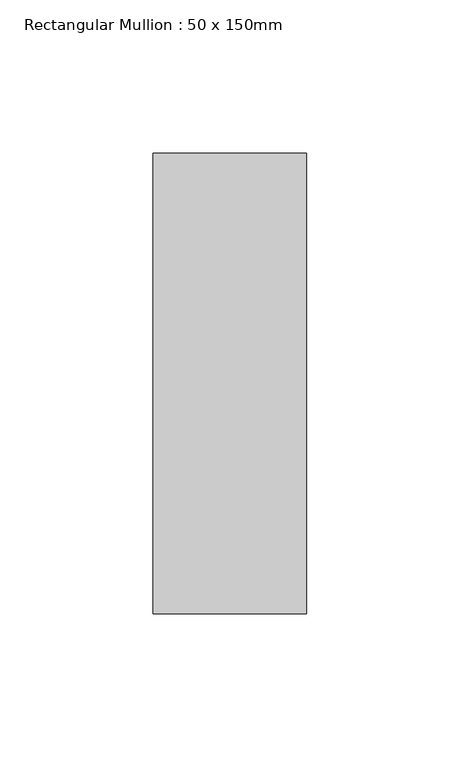
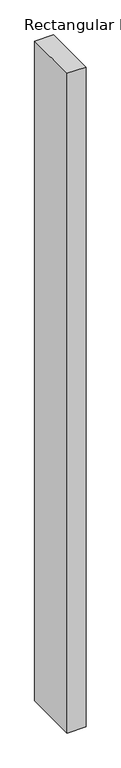
"""IFC4 building model written with IfcOpenShell, lengths in millimetres: member geometry, Rectangular Mullion : 50 x 150mm."""

from ifc_helpers import new_model, si_unit, frame, origin, place, context, project, spatial, polyline, outline, extrude, source, transform, mapped, element, save


def rectangular_mullion_50_x_150mm_17218063(model_context):
    return source(origin(), model_context, "Body", "SweptSolid", [
        extrude(outline(polyline([(0.0, 75.0), (0.0, -75.0), (-50.0, -75.0), (-50.0, 75.0), (0.0, 75.0)])), frame((0.0, 0.0, -1855.0), z_axis=(0.0, 0.0, 1.0), x_axis=(1.0, 0.0, 0.0)), (0.0, 0.0, 1.0), 1855.0),
    ])


if __name__ == "__main__":
    model = new_model("IFC4")
    model_context = context("Model", 3, world=origin())
    ifc_project = project(units=[si_unit("LENGTHUNIT", "METRE", prefix="MILLI")], contexts=[model_context])
    site = spatial("IfcSite", under=ifc_project)
    building = spatial("IfcBuilding", under=site)
    placement = place(None, origin())
    rectangular_mullion_50_x_150mm_shape = rectangular_mullion_50_x_150mm_17218063(model_context)
    element("IfcMember", 1, ObjectType="Rectangular Mullion : 50 x 150mm", at=placement, inside=building, context=model_context, shape_type="MappedRepresentation", body=[
        mapped(rectangular_mullion_50_x_150mm_shape, transform((0.0, 0.0, 0.0), x_axis=(1.0, 0.0, 0.0), y_axis=(0.0, 1.0, 0.0), z_axis=(0.0, 0.0, 1.0))),
    ])
    save(model, "model.ifc")

# Revit data of these elements
# Type "Rectangular Mullion : 50 x 150mm"
#   built-in parameter 1007304 = 0.492126 (stored number, unit not read)
#   built-in parameter 1007301 = 0.082021 (stored number, unit not read)
#   built-in parameter 1007300 = 0.082021 (stored number, unit not read)
# Element 1 (IfcMember, "Rectangular Mullion : 50 x 150mm")
#   Materials on its faces: "Aluminium"
# Materials
#   "Aluminium": class "Metal", colour RGB 247 247 247, transparency 0, Description = "Aluminium 6061", Cost = 0
